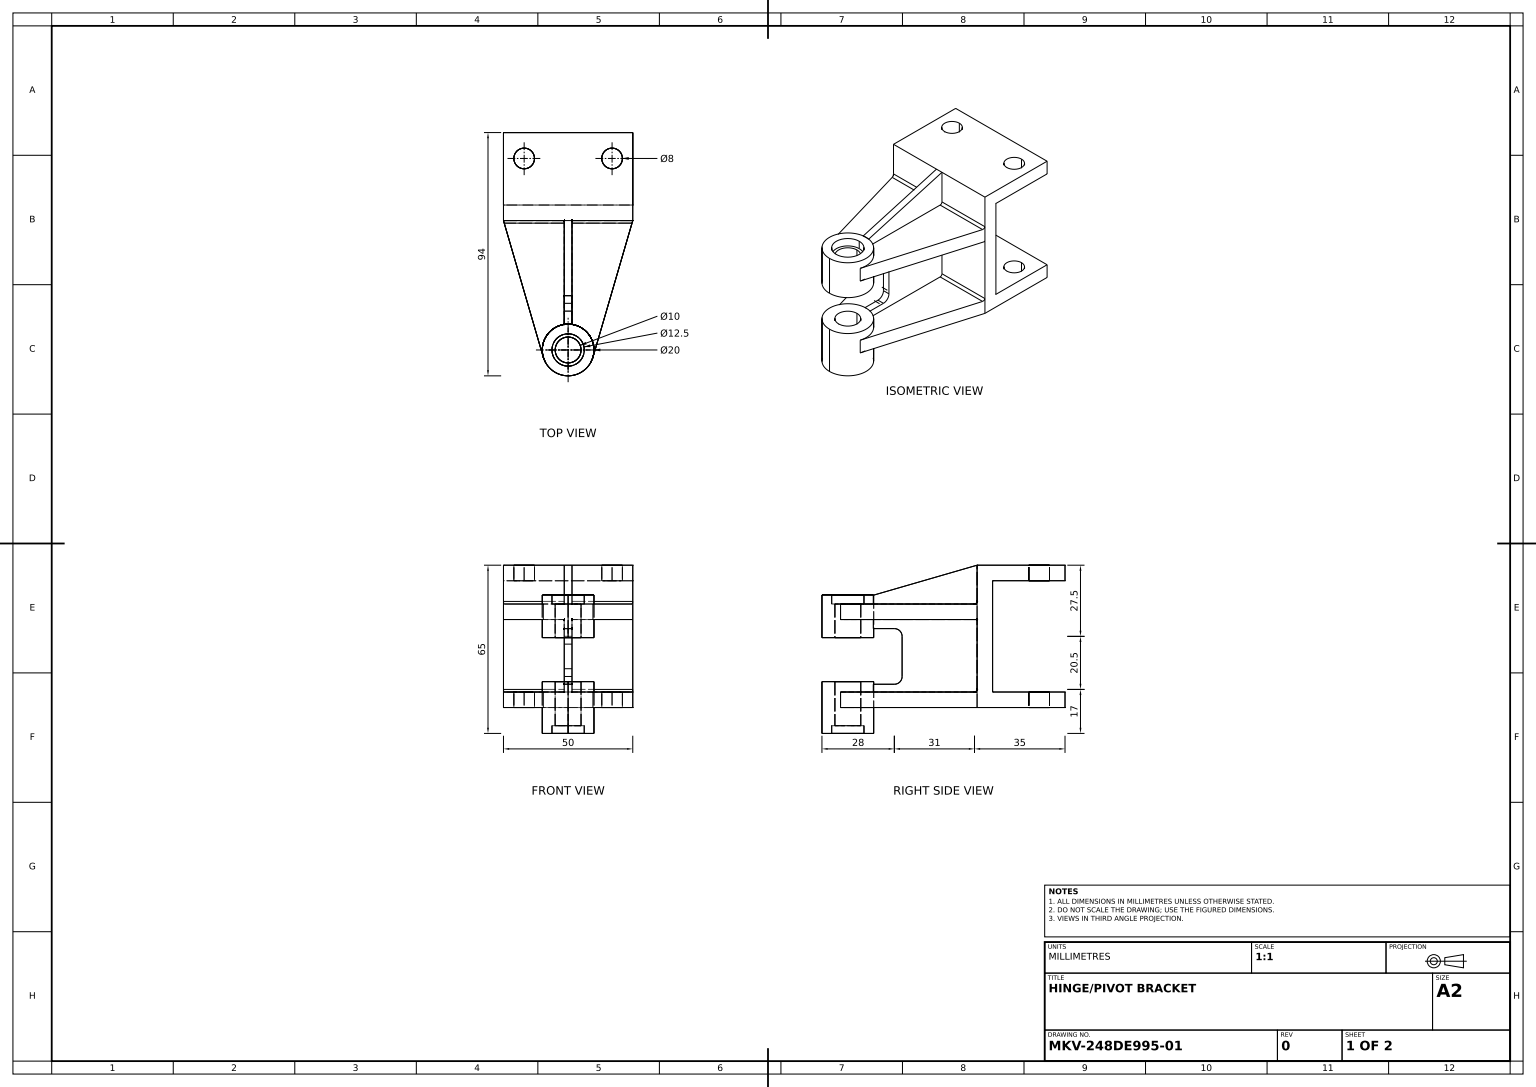
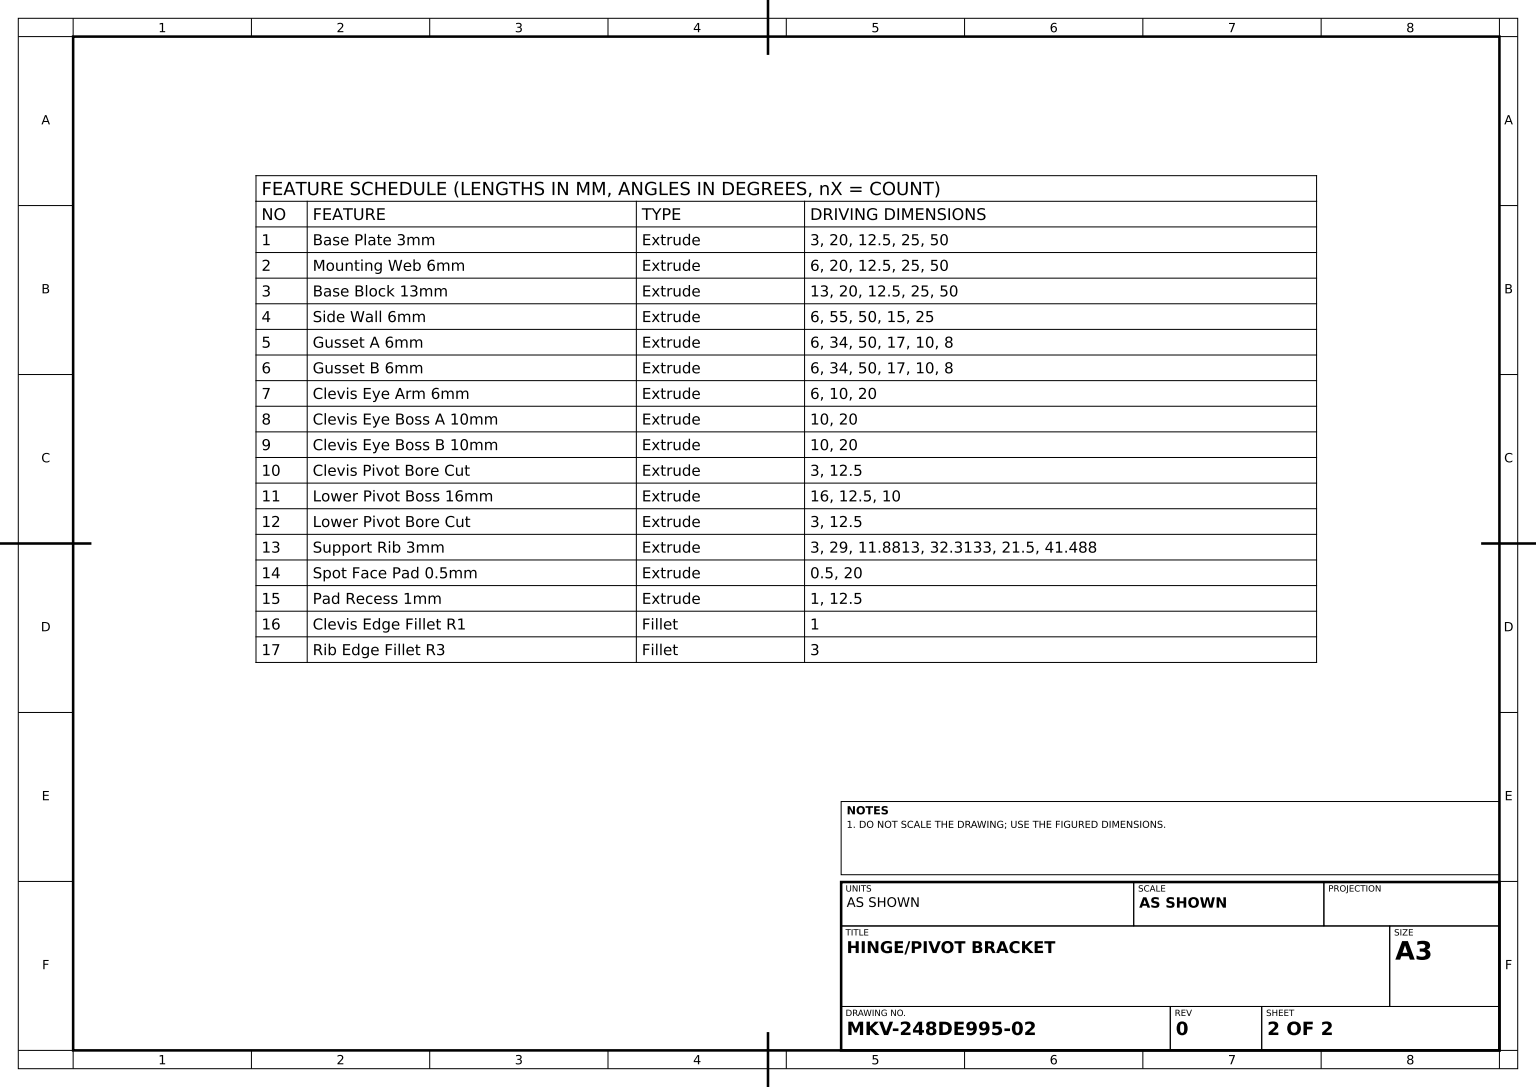
from build123d import *

# Parameters (mm, degrees)
BASE_PROFILE_SKETCH_R        = 10
BASE_PROFILE_SKETCH_R_2      = 6.25
BASE_PLATE_3MM_DEPTH         = 3
MOUNTING_WEB_6MM_DEPTH       = 6
BASE_START                   = -13
SKETCH1_4_R                  = 10
SKETCH1_4_R_2                = 6.25
BASE_BLOCK_13MM_DEPTH        = 13
SIDE_WALL_SKETCH_W           = 50
SIDE_WALL_SKETCH_H           = 55
SIDE_WALL_6MM_DEPTH          = 6
GUSSET_PROFILE_SKETCH_W      = 50
GUSSET_PROFILE_SKETCH_H      = 34
GUSSET_PROFILE_SKETCH_R      = 4
GUSSET_A_6MM_DEPTH           = 6
GUSSET_START                 = -49
SKETCH3_2_W                  = 50
SKETCH3_2_H                  = 34
SKETCH3_2_R                  = 4
GUSSET_B_6MM_DEPTH           = 6
CLEVIS_EYE_SKETCH_R          = 10
CLEVIS_EYE_SKETCH_R_2        = 5
CLEVIS_EYE_ARM_6MM_DEPTH     = 6
SKETCH4_3_R                  = 10
SKETCH4_3_R_2                = 5
CLEVIS_EYE_BOSS_A_10MM_DEPTH = 10
CLEVIS_START                 = 10
SKETCH4_4_R                  = 10
SKETCH4_4_R_2                = 5
CLEVIS_EYE_BOSS_B_10MM_DEPTH = 10
CLEVIS_PIVOT_BORE_SKETCH_R   = 6.25
CLEVIS_PIVOT_BORE_CUT_DEPTH  = 3
LOWER_PIVOT_BOSS_SKETCH_R    = 6.25
LOWER_PIVOT_BOSS_SKETCH_R_2  = 5
LOWER_PIVOT_BOSS_16MM_DEPTH  = 16
LOWER_START                  = -3
LOWER_PIVOT_BORE_SKETCH_R    = 6.25
LOWER_PIVOT_BORE_CUT_DEPTH   = 3
SUPPORT_RIB_3MM_DEPTH        = 1.5
SPOT_FACE_PAD_SKETCH_R       = 10
SPOT_FACE_PAD_0_5MM_DEPTH    = 0.5
PAD_START                    = -1
PAD_RECESS_SKETCH_R          = 6.25
PAD_RECESS_1MM_DEPTH         = 1
CLEVIS_EDGE_FILLET_R1_R      = 1
RIB_EDGE_FILLET_R3_R         = 3


with BuildPart() as part:
    # Base Profile Sketch → Base Plate 3mm (new body)
    with BuildSketch(Plane(origin=(0, 0, 0), x_dir=(1, 0, 0), z_dir=(0, 1, 0))):
        with Locations(Location((0, 0, 0), (0, 0, 270))):
            Circle(BASE_PROFILE_SKETCH_R)
        with Locations(Location((0, 0, 0), (0, 0, 270))):
            Circle(BASE_PROFILE_SKETCH_R_2, mode=Mode.SUBTRACT)
    extrude(amount=BASE_PLATE_3MM_DEPTH)



with BuildPart() as body_2:
    # Sketch1_3 → Mounting Web 6mm (new body)
    with BuildSketch(Plane(origin=(0, 0, 0), x_dir=(1, 0, 0), z_dir=(0, 1, 0))):
        with BuildLine():
            Line((25, 50), (-25, 50))
            Line((-25, 50), (-9.6, -2.8))
            ThreePointArc((-9.6, -2.8), (-1.414213562, 9.899494937), (10, 0))
            ThreePointArc((10, 0), (9.899494937, -1.414213562), (9.6, -2.8))
            Line((9.6, -2.8), (25, 50))
        make_face()
    extrude(amount=-MOUNTING_WEB_6MM_DEPTH)


with BuildPart() as part_1:
    add(part.part)

    add(body_2.part)  # Base Block 13mm merges body 2
    # Sketch1_4 → Base Block 13mm (add)
    with BuildSketch(Plane(origin=(0, 0, 0), x_dir=(1, 0, 0), z_dir=(0, 1, 0)).offset(BASE_START)):
        with Locations(Location((0, 0, 0), (0, 0, 270))):
            Circle(SKETCH1_4_R)
        with Locations(Location((0, 0, 0), (0, 0, 270))):
            Circle(SKETCH1_4_R_2, mode=Mode.SUBTRACT)
    extrude(amount=BASE_BLOCK_13MM_DEPTH)

    # Side Wall Sketch → Side Wall 6mm (add)
    with BuildSketch(Plane(origin=(0, 0, -50), x_dir=(-1, 0, 0), z_dir=(0, 0, -1))):
        with Locations((0, -12.5)):
            Rectangle(SIDE_WALL_SKETCH_W, SIDE_WALL_SKETCH_H)
    extrude(amount=SIDE_WALL_6MM_DEPTH)

    # Gusset Profile Sketch → Gusset A 6mm (add)
    with BuildSketch(Plane(origin=(0, 15, 0), x_dir=(1, 0, 0), z_dir=(0, 1, 0))):
        with Locations((0, 67)):
            Rectangle(GUSSET_PROFILE_SKETCH_W, GUSSET_PROFILE_SKETCH_H)
        with Locations(Location((-17, 74, 0), (0, 0, 270))):
            Circle(GUSSET_PROFILE_SKETCH_R, mode=Mode.SUBTRACT)
        with Locations(Location((17, 74, 0), (0, 0, 270))):
            Circle(GUSSET_PROFILE_SKETCH_R, mode=Mode.SUBTRACT)
    extrude(amount=-GUSSET_A_6MM_DEPTH)

    # Sketch3_2 → Gusset B 6mm (add)
    with BuildSketch(Plane(origin=(0, 15, 0), x_dir=(1, 0, 0), z_dir=(0, 1, 0)).offset(GUSSET_START)):
        with Locations((0, 67)):
            Rectangle(SKETCH3_2_W, SKETCH3_2_H)
        with Locations(Location((-17, 74, 0), (0, 0, 270))):
            Circle(SKETCH3_2_R, mode=Mode.SUBTRACT)
        with Locations(Location((17, 74, 0), (0, 0, 270))):
            Circle(SKETCH3_2_R, mode=Mode.SUBTRACT)
    extrude(amount=-GUSSET_B_6MM_DEPTH)

    # Clevis Eye Sketch → Clevis Eye Arm 6mm (add)
    # profile 1 of 2: a face of its own
    with BuildSketch(Plane.XZ.offset(40)):
        with BuildLine():
            Line((-9.6, 2.8), (-25, -50))
            Line((-25, -50), (25, -50))
            Line((25, -50), (9.6, 2.8))
            ThreePointArc((9.6, 2.8), (9.899494937, 1.414213562), (10, 0))
            ThreePointArc((10, 0), (-1.414213562, -9.899494937), (-9.6, 2.8))
        make_face()
    # profile 2 of 2: a face of its own
    with BuildSketch(Plane.XZ.offset(40)):
        with Locations(Location((0, 0, 0), (0, 0, 90))):
            Circle(CLEVIS_EYE_SKETCH_R)
        with Locations(Location((0, 0, 0), (0, 0, 270))):
            Circle(CLEVIS_EYE_SKETCH_R_2, mode=Mode.SUBTRACT)
    extrude(amount=-CLEVIS_EYE_ARM_6MM_DEPTH)

    # Sketch4_3 → Clevis Eye Boss A 10mm (add)
    with BuildSketch(Plane.XZ.offset(40)):
        with Locations(Location((0, 0, 0), (0, 0, 90))):
            Circle(SKETCH4_3_R)
        with Locations(Location((0, 0, 0), (0, 0, 270))):
            Circle(SKETCH4_3_R_2, mode=Mode.SUBTRACT)
    extrude(amount=-CLEVIS_EYE_BOSS_A_10MM_DEPTH)

    # Sketch4_4 → Clevis Eye Boss B 10mm (add)
    with BuildSketch(Plane.XZ.offset(40).offset(CLEVIS_START)):
        with Locations(Location((0, 0, 0), (0, 0, 90))):
            Circle(SKETCH4_4_R)
        with Locations(Location((0, 0, 0), (0, 0, 270))):
            Circle(SKETCH4_4_R_2, mode=Mode.SUBTRACT)
    extrude(amount=-CLEVIS_EYE_BOSS_B_10MM_DEPTH)

    # Clevis Pivot Bore Sketch → Clevis Pivot Bore Cut (cut)
    with BuildSketch(Plane.XZ.offset(50)):
        with Locations(Location((0, 0, 0), (0, 0, 90))):
            Circle(CLEVIS_PIVOT_BORE_SKETCH_R)
    extrude(amount=-CLEVIS_PIVOT_BORE_CUT_DEPTH, mode=Mode.SUBTRACT)

    # Lower Pivot Boss Sketch → Lower Pivot Boss 16mm (add)
    with BuildSketch(Plane.XZ.offset(13)):
        with Locations(Location((0, 0, 0), (0, 0, 270))):
            Circle(LOWER_PIVOT_BOSS_SKETCH_R)
        with Locations(Location((0, 0, 0), (0, 0, 270))):
            Circle(LOWER_PIVOT_BOSS_SKETCH_R_2, mode=Mode.SUBTRACT)
    extrude(amount=-LOWER_PIVOT_BOSS_16MM_DEPTH)

    # Lower Pivot Bore Sketch → Lower Pivot Bore Cut (cut)
    with BuildSketch(Plane(origin=(0, 3, 0), x_dir=(1, 0, 0), z_dir=(0, 1, 0)).offset(LOWER_START)):
        with Locations(Location((0, 0, 0), (0, 0, 90))):
            Circle(LOWER_PIVOT_BORE_SKETCH_R)
    extrude(amount=LOWER_PIVOT_BORE_CUT_DEPTH, mode=Mode.SUBTRACT)

    # Support Rib Sketch → Support Rib 3mm (add, symmetric)
    with BuildSketch(Plane(origin=(0, 0, 0), x_dir=(0, 0, -1), z_dir=(1, 0, 0))):
        Polygon((50, 15), (8.511959117, 3), (8.511959117, 0), (50, 0), align=None)
        Polygon((9.118743045, -9.5), (21, -9.5), (21, -31), (9.118743045, -31), (9.118743045, -34), (50, -34), (50, -6), (9.118743045, -6), align=None)
    extrude(amount=SUPPORT_RIB_3MM_DEPTH, both=True)

    # Spot Face Pad Sketch → Spot Face Pad 0.5mm (add)
    with BuildSketch(Plane(origin=(0, 3, 0), x_dir=(1, 0, 0), z_dir=(0, 1, 0))):
        with Locations(Location((0, 0, 0), (0, 0, 270))):
            Circle(SPOT_FACE_PAD_SKETCH_R)
    extrude(amount=SPOT_FACE_PAD_0_5MM_DEPTH)

    # Pad Recess Sketch → Pad Recess 1mm (cut)
    with BuildSketch(Plane(origin=(0, 3.5, 0), x_dir=(1, 0, 0), z_dir=(0, 1, 0)).offset(PAD_START)):
        with Locations(Location((0, 0, 0), (0, 0, 90))):
            Circle(PAD_RECESS_SKETCH_R)
    extrude(amount=PAD_RECESS_1MM_DEPTH, mode=Mode.SUBTRACT)

    # Clevis Edge Fillet R1
    clevis_edge_fillet_r1_edges = [part_1.edges().sort_by_distance(p)[0] for p in [
        (13.25, 0, -50),
        (-13.25, 0, -50),
        (-13.25, -34, -50),
        (13.25, -34, -50),
    ]]
    fillet(clevis_edge_fillet_r1_edges, radius=CLEVIS_EDGE_FILLET_R1_R)

    # Rib Edge Fillet R3
    rib_edge_fillet_r3_edges = [part_1.edges().sort_by_distance(p)[0] for p in [
        (0, -9.5, -21),
        (0, -31, -21),
    ]]
    fillet(rib_edge_fillet_r3_edges, radius=RIB_EDGE_FILLET_R3_R)


solid = part_1.part
